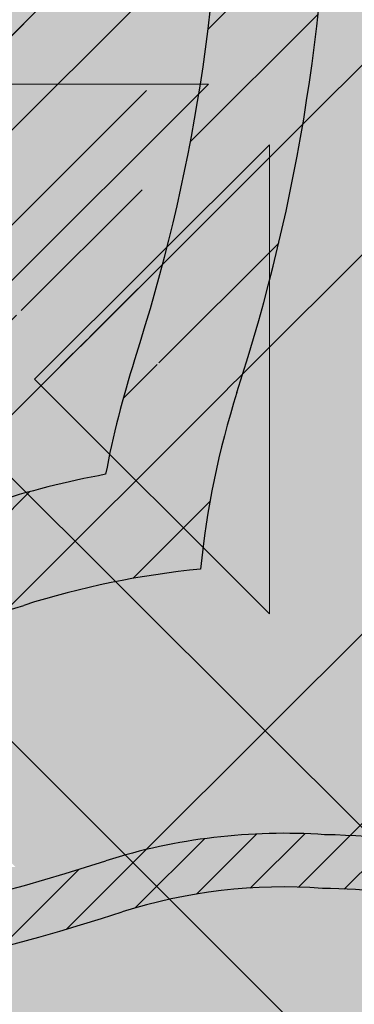
# Model space of a CAD drawing. Units: inches. Extents: x 844 to 2234, y 346 to 1084.
# Tile 10 of 93: x 1124.57 to 1125.562, y 688.258 to 691.183. Entities that reach past the tile are written whole.
import ezdxf

# ---------------------------------------------------------------- set-up
doc = ezdxf.new("R2010")
doc.units = ezdxf.units.IN
doc.header["$MEASUREMENT"] = 0
for name, color, linetype, lineweight in [('A-ANNO-DIMS', 2, 'Continuous', 18), ('furniture', 8, 'Continuous', 18), ('RA-AP-01$0$INT', 35, 'Continuous', 5)]:
    doc.layers.add(name, color=color, linetype=linetype, lineweight=lineweight)
doc.layers.add('RA-AP-01$0$FURN', color=3, linetype='Continuous')
doc.layers.add('RA-AP-01$0$WOOD', color=64, linetype='Continuous')
doc.styles.get("Standard").update_dxf_attribs({"font": 'arial.ttf'})
doc.dimstyles.get("Standard").update_dxf_attribs({"dimtxt": 6, "dimasz": 3, "dimexe": 0.18, "dimexo": 0.0625, "dimgap": 0.09, "dimtad": 0, "dimtih": 1, "dimtoh": 1, "dimdec": 1, "dimzin": 0, "dimdsep": 46, "dimlunit": 3, "dimtxsty": 'Standard', "dimblk": 'ARCHTICK', "dimcen": 0.09, "dimadec": 0, "dimazin": 0, "dimtfac": 1, "dimtdec": 1, "dimtofl": 0, "dimtmove": 0, "dimatfit": 3, "dimfxl": 1, "dimtolj": 1, "dimtzin": 0, "dimarcsym": 0})

# ---------------------------------------------------------------- blocks, each defined once
blk = doc.blocks.new('A$C18D01794')
at = {"layer": 'RA-AP-01$0$INT'}
h = blk.add_hatch(color=256, dxfattribs=at)
h.paths.add_polyline_path([(4.585917135068449, -6.356712009588271), (4.555206456959269, -6.35671200958746), (4.555206456959137, -6.387422687716308), (4.874495778835233, -6.706712009592356), (4.90520645695423, -6.676001331474049)])
h.paths.add_polyline_path([(5.255206456948813, -6.387422687716306), (5.255206456948682, -6.356712009605972), (5.224495778822613, -6.356712009605161), (4.905206456953498, -6.676001331474273), (4.935917135072151, -6.706712009592924)])
h.paths.add_polyline_path([(4.935917135072559, -6.706712009592068), (4.905206456953564, -6.737422687710376), (5.255206456951813, -7.087422687708613), (5.255206456951549, -7.026001331471008)])
h.paths.add_polyline_path([(4.555206456956399, -7.026001331471013), (4.555206456956134, -7.087422687708616), (4.905206456953821, -6.737422687710943), (4.874495778835166, -6.70671200959229)])
h = blk.add_hatch(color=256, dxfattribs=at)
h.paths.add_polyline_path([(4.585917135068448, -6.356712009588273), (4.614201406330596, -6.356712009589021), (4.668846067270487, -6.411356670531338), (4.723490728212344, -6.356712009591912), (4.771774999457151, -6.35671200959319), (4.826419660396886, -6.411356670535356), (4.862780050090322, -6.374996280843536), (4.844495778842715, -6.356712009595112), (4.862780050090411, -6.356712009595595), (4.905206456960182, -6.399138416468211), (4.947632863832445, -6.356712009597838), (4.965917135079675, -6.356712009598322), (4.947632863831759, -6.374996280845421), (4.983993253523576, -6.411356670538857), (5.038637914464627, -6.356712009600247), (5.08692218571208, -6.356712009601523), (5.141566846649976, -6.411356670541852), (5.196211507589851, -6.356712009604411), (5.224495778822615, -6.356712009605161), (4.905206456953975, -6.676001331473793)])
h.paths.add_polyline_path([(4.895206456956031, -6.637717060225675), (4.895206456958921, -6.528427738347902), (4.840561796018589, -6.583072399285802)], flags=16)
h.paths.add_polyline_path([(4.915206456955638, -6.637717060226121), (4.969851117895509, -6.583072399288678), (4.915206456957609, -6.528427738348344)], flags=16)
h.paths.add_polyline_path([(4.826419660395175, -6.568930263661755), (4.881064321335613, -6.514285602723745), (4.771774999456703, -6.514285602720857)], flags=16)
h.paths.add_polyline_path([(4.983993253519558, -6.568930263665262), (5.038637914460456, -6.514285602726792), (4.929348592581548, -6.514285602724816)], flags=16)
h.paths.add_polyline_path([(4.881064321336025, -6.494285602723742), (4.826419660397532, -6.439640941782821), (4.771774999457062, -6.494285602720859)], flags=16)
h.paths.add_polyline_path([(4.929348592582019, -6.494285602724817), (5.038637914460982, -6.494285602726792), (4.983993253522945, -6.439640941786327)], flags=16)
h.paths.add_polyline_path([(4.895206456960191, -6.480143467100443), (4.895206456962115, -6.407422687715913), (4.876922185715016, -6.389138416467584), (4.840561796021581, -6.425498806159401)], flags=16)
h.paths.add_polyline_path([(4.915206456958487, -6.480143467100889), (4.969851117899527, -6.425498806162279), (4.933490728206909, -6.389138416468043), (4.9152064569598, -6.40742268771434)], flags=16)
h.paths.add_polyline_path([(4.757632863832376, -6.480143467096812), (4.812277524772842, -6.425498806158772), (4.757632863834348, -6.370854145217844)], flags=16)
h.paths.add_polyline_path([(4.737632863832376, -6.480143467096286), (4.737632863834348, -6.370854145217375), (4.682988202893906, -6.425498806155385)], flags=16)
h.paths.add_polyline_path([(5.05278005008503, -6.480143467103376), (5.052780050087917, -6.370854145224413), (4.998135389146995, -6.425498806162908)], flags=16)
h.paths.add_polyline_path([(5.072780050085024, -6.480143467103744), (5.127424711025931, -6.42549880616527), (5.072780050087916, -6.370854145224832)], flags=16)
h.paths.add_polyline_path([(4.935917135072783, -6.706712009592292), (5.255206456948811, -6.387422687716309), (5.255206456948932, -6.415706958964177), (5.200561796010279, -6.470351619902839), (5.255206456949403, -6.524996280841948), (5.25520645694961, -6.5732805520894), (5.200561796009787, -6.627925213029239), (5.236922185702417, -6.664285602721864), (5.255206456949919, -6.646001331474357), (5.255206456949998, -6.664285602721898), (5.212780050078687, -6.706712009592262), (5.25520645695036, -6.749138416463932), (5.255206456950438, -6.767422687711313), (5.236922185702424, -6.749138416463297), (5.200561796009796, -6.785498806155928), (5.255206456950753, -6.840143467096874), (5.25520645695096, -6.888427738341682), (5.200561796010322, -6.943072399282328), (5.255206456951428, -6.997717060223427), (5.255206456951547, -7.026001331471006)])
h.paths.add_polyline_path([(5.042988202883395, -6.785498806155427), (5.097632863823085, -6.840143467095101), (5.097632863822622, -6.730854145216193)], flags=16)
h.paths.add_polyline_path([(5.028846067259663, -6.771356670531693), (5.083490728198774, -6.716712009592573), (4.974201406321001, -6.716712009593042)], flags=16)
h.paths.add_polyline_path([(5.117632863823087, -6.840143467095186), (5.172277524762331, -6.785498806155926), (5.11763286382262, -6.730854145216225)], flags=16)
h.paths.add_polyline_path([(5.08349072819877, -6.696712009593886), (5.028846067259652, -6.642067348654775), (4.974201406320998, -6.696712009593438)], flags=16)
h.paths.add_polyline_path([(5.131774999446817, -6.854285602718917), (5.186419660386065, -6.799640941779662), (5.241064321325782, -6.854285602719365)], flags=17)
h.paths.add_polyline_path([(5.131774999446228, -6.716712009592374), (5.186419660386065, -6.771356670532194), (5.222780050079488, -6.734996280838764), (5.204495778832781, -6.716712009592063)], flags=16)
h.paths.add_polyline_path([(5.097632863822613, -6.682569873970264), (5.097632863823061, -6.573280552091354), (5.042988202883383, -6.627925213031044)], flags=16)
h.paths.add_polyline_path([(5.131774999446899, -6.874285602718915), (5.241064321325809, -6.874285602719364), (5.186419660386591, -6.928930263658598)], flags=17)
h.paths.add_polyline_path([(5.131774999446226, -6.696712009594078), (5.204495778830767, -6.696712009594374), (5.22278005007868, -6.67842773834687), (5.186419660386049, -6.642067348654249)], flags=16)
h.paths.add_polyline_path([(5.11763286382262, -6.682569873970225), (5.17227752476232, -6.627925213030515), (5.117632863823064, -6.573280552091267)], flags=16)
h.paths.add_polyline_path([(5.186419660386069, -6.613783077405491), (5.241064321325754, -6.559138416465795), (5.131774999446791, -6.559138416466263)], flags=16)
h.paths.add_polyline_path([(5.131774999446872, -6.539138416466263), (5.24106432132578, -6.539138416465794), (5.186419660386554, -6.484493755526573)], flags=16)
h.paths.add_polyline_path([(5.255206456951811, -7.08742268770861), (5.255206456951895, -7.106712009588038), (4.555206456956052, -7.106712009588038), (4.555206456956136, -7.087422687708617), (4.905206456953973, -6.737422687710788)])
h.paths.add_polyline_path([(4.983993253513404, -6.8444937555241), (4.92934859257295, -6.899138416462108), (5.03863791445186, -6.899138416465014)], flags=16)
h.paths.add_polyline_path([(4.969851117889988, -6.83035161990006), (4.915206456952556, -6.775706958960171), (4.915206456949648, -6.884996280837944)], flags=16)
h.paths.add_polyline_path([(4.929348592572535, -6.919138416462105), (4.983993253511019, -6.973783077403037), (5.038637914451496, -6.919138416465012)], flags=16)
h.paths.add_polyline_path([(5.052780050074912, -6.93328055208906), (4.998135389134438, -6.987925213027088), (5.052780050072919, -7.042569873968025)], flags=16)
h.paths.add_polyline_path([(5.07278005007491, -6.933280552089588), (5.072780050072918, -7.042569873968497), (5.127424711013374, -6.987925213030498)], flags=16)
h.paths.add_polyline_path([(4.89520645695295, -6.775706958959721), (4.840561796013067, -6.830351619897157), (4.895206456950961, -6.884996280837494)], flags=16)
h.paths.add_polyline_path([(4.915206456948365, -6.933280552085403), (4.915206456946434, -7.006001331471951), (4.933490728192729, -7.024285602719066), (4.969851117886972, -6.987925213026453)], flags=16)
h.paths.add_polyline_path([(4.881064321327021, -6.899138416461022), (4.82641966038902, -6.84449375552057), (4.771774999448108, -6.899138416459029)], flags=16)
h.paths.add_polyline_path([(4.895206456950073, -6.933280552084951), (4.840561796009022, -6.987925213023558), (4.876922185700835, -7.024285602716997), (4.895206456948749, -7.006001331469487)], flags=16)
h.paths.add_polyline_path([(4.983993253510392, -7.0020673486505), (4.947632863816944, -7.038427738342319), (4.965917135064043, -7.05671200959023), (5.038637914448995, -7.056712009591555)], flags=16)
h.paths.add_polyline_path([(4.881064321326543, -6.91913841646102), (4.771774999447578, -6.919138416459031), (4.826419660385607, -6.973783077399508)], flags=16)
h.paths.add_polyline_path([(4.905206456946447, -7.014285602717636), (4.862780050074785, -7.056712009588352), (4.947632863816685, -7.056712009589775)], flags=16)
h.paths.add_polyline_path([(5.14156684663679, -7.002067348654549), (5.086922185696452, -7.056712009592438), (5.196211507574223, -7.056712009594425)], flags=16)
h.paths.add_polyline_path([(4.8264196603837, -7.002067348646972), (4.771774999442643, -7.056712009585575), (4.8444957788276, -7.056712009587508), (4.862780050075511, -7.038427738340416)], flags=16)
h.paths.add_polyline_path([(4.812277524760289, -6.98792521302292), (4.757632863822258, -6.933280552082447), (4.757632863819352, -7.042569873961408)], flags=16)
h.paths.add_polyline_path([(4.73763286382226, -6.933280552082079), (4.682988202881349, -6.987925213020536), (4.737632863819352, -7.04256987396099)], flags=16)
h.paths.add_polyline_path([(4.723490728195188, -7.056712009584289), (4.668846067257299, -7.002067348643949), (4.614201406317417, -7.056712009581383)], flags=16)
h.paths.add_polyline_path([(4.597632863829262, -6.706712009592262), (4.555206456957951, -6.664285602721896), (4.555206456958029, -6.646001331474357), (4.573490728205535, -6.664285602721864), (4.609851117898167, -6.627925213029238), (4.555206456958338, -6.573280552089402), (4.555206456958546, -6.524996280841952), (4.60985111789767, -6.470351619902839), (4.555206456959015, -6.415706958964177), (4.555206456959138, -6.387422687716309), (4.874495778835167, -6.70671200959229), (4.5552064569564, -7.026001331471015), (4.555206456956523, -6.997717060223433), (4.609851117897629, -6.94307239928233), (4.555206456956988, -6.888427738341681), (4.555206456957198, -6.840143467096881), (4.609851117898153, -6.78549880615593), (4.573490728205528, -6.749138416463297), (4.555206456957507, -6.76742268771132), (4.555206456957585, -6.749138416463933)])
h.paths.add_polyline_path([(4.712780050085332, -6.730854145216195), (4.712780050084863, -6.840143467095105), (4.767424711024555, -6.785498806155427)], flags=16)
h.paths.add_polyline_path([(4.726922185709173, -6.716712009592573), (4.781566846648288, -6.771356670531693), (4.836211507586949, -6.716712009593043)], flags=16)
h.paths.add_polyline_path([(4.692780050085327, -6.730854145216225), (4.638135389145619, -6.785498806155928), (4.692780050084865, -6.840143467095185)], flags=16)
h.paths.add_polyline_path([(4.726922185709182, -6.696712009593886), (4.836211507586949, -6.696712009593436), (4.7815668466483, -6.642067348654773)], flags=16)
h.paths.add_polyline_path([(4.678637914461726, -6.71671200959237), (4.605917135075169, -6.716712009592063), (4.587632863828464, -6.734996280838766), (4.623993253521887, -6.771356670532195)], flags=16)
h.paths.add_polyline_path([(4.712780050085336, -6.68256987397026), (4.767424711024568, -6.627925213031042), (4.71278005008489, -6.573280552091352)], flags=16)
h.paths.add_polyline_path([(4.678637914461726, -6.696712009594076), (4.623993253521899, -6.642067348654247), (4.587632863829271, -6.67842773834687), (4.605917135077185, -6.696712009594376)], flags=16)
h.paths.add_polyline_path([(4.692780050085336, -6.682569873970228), (4.692780050084889, -6.573280552091267), (4.638135389145632, -6.627925213030515)], flags=16)
h.paths.add_polyline_path([(4.623993253521885, -6.799640941779662), (4.678637914461131, -6.854285602718915), (4.56934859258217, -6.854285602719365)], flags=17)
h.paths.add_polyline_path([(4.623993253521901, -6.613783077405509), (4.678637914461158, -6.559138416466263), (4.569348592582195, -6.559138416465795)], flags=16)
h.paths.add_polyline_path([(4.678637914461051, -6.874285602718915), (4.623993253521361, -6.928930263658598), (4.569348592582143, -6.874285602719364)], flags=17)
h.paths.add_polyline_path([(4.678637914461076, -6.539138416466263), (4.623993253521399, -6.484493755526573), (4.569348592582167, -6.539138416465796)], flags=16)
h = blk.add_hatch(color=256, dxfattribs=at)
h.paths.add_polyline_path([(5.028846067259997, -6.642067348655121), (4.974201406321342, -6.696712009593783), (5.083490728199115, -6.69671200959423)])
h.paths.add_polyline_path([(4.974201406321344, -6.716712009593388), (5.028846067260004, -6.771356670532039), (5.083490728199117, -6.716712009592919)])
h.paths.add_polyline_path([(5.042988202883738, -6.785498806155768), (5.097632863823428, -6.840143467095449), (5.097632863822963, -6.73085414521654)])
h.paths.add_polyline_path([(5.117632863822961, -6.730854145216568), (5.117632863823428, -6.840143467095531), (5.172277524762674, -6.785498806156272)])
h.paths.add_polyline_path([(5.131774999446572, -6.716712009592718), (5.186419660386406, -6.77135667053254), (5.222780050079831, -6.734996280839116), (5.204495778833122, -6.716712009592409)])
h.paths.add_polyline_path([(5.236922185702764, -6.749138416463644), (5.200561796010139, -6.785498806156274), (5.255206456949971, -6.840143467096101), (5.255206456950271, -6.76742268771115)])
h.paths.add_polyline_path([(5.186419660386412, -6.799640941780006), (5.131774999447164, -6.854285602719262), (5.241064321326123, -6.854285602719711)])
h.paths.add_polyline_path([(5.131774999447238, -6.874285602719261), (5.186419660386934, -6.928930263658944), (5.241064321326153, -6.874285602719709)])
h.paths.add_polyline_path([(5.200561796010663, -6.943072399282675), (5.255206456949324, -6.997717060221329), (5.255206456949777, -6.888427738343558)])
h.paths.add_polyline_path([(5.21278005007903, -6.706712009592607), (5.255206456950223, -6.749138416463798), (5.255206456950696, -6.664285602721891)])
h.paths.add_polyline_path([(5.13177499944657, -6.696712009594424), (5.204495778831106, -6.696712009594723), (5.222780050079024, -6.678427738347219), (5.186419660386397, -6.642067348654592)])
h.paths.add_polyline_path([(5.117632863823405, -6.573280552091611), (5.117632863822955, -6.682569873970578), (5.172277524762665, -6.627925213030859)])
h.paths.add_polyline_path([(5.042988202883727, -6.627925213031387), (5.097632863822957, -6.682569873970603), (5.097632863823407, -6.573280552091697)])
h.paths.add_polyline_path([(5.131774999447135, -6.559138416466609), (5.186419660386394, -6.613783077405857), (5.241064321326097, -6.559138416466144)])
h.paths.add_polyline_path([(5.200561796010128, -6.627925213029584), (5.236922185702758, -6.664285602722211), (5.255206456950264, -6.646001331474705), (5.255206456949948, -6.573280552089752)])
h.paths.add_polyline_path([(5.186419660386895, -6.484493755526919), (5.131774999447213, -6.539138416466609), (5.241064321326127, -6.539138416466142)])
h.paths.add_polyline_path([(5.200561796010624, -6.470351619903183), (5.255206456949745, -6.524996280842298), (5.255206456949276, -6.415706958964523)])
for p, q in [((4.905206456953975, -6.676001331473793), (5.224495778822613, -6.356712009605161)), ((4.935917135072783, -6.706712009592292), (5.255206456948813, -6.387422687716307)), ((5.042988202883385, -6.627925213031041), (5.097632863823062, -6.573280552091352)), ((5.097632863823062, -6.573280552091352), (5.097632863822615, -6.682569873970262)), ((5.097632863822615, -6.682569873970262), (5.042988202883383, -6.627925213031042)), ((5.083490728198769, -6.696712009593882), (5.028846067259652, -6.642067348654775)), ((5.08349072819877, -6.696712009593886), (4.974201406320999, -6.696712009593436))]:
    blk.add_line(p, q, dxfattribs=at)
blk = doc.blocks.new('A$C32926AE1')
at = {"layer": 'RA-AP-01$0$FURN'}
h = blk.add_hatch(dxfattribs=at)
h.set_pattern_fill('ANSI31', color=256, scale=0.1, style=0)
h.set_pattern_definition([(45, (0, 0), (-0.0088388347648318, 0.0088388347648318), [])])
edge = h.paths.add_edge_path(flags=16)
edge.add_arc((4.904771284329206, 4.246793130718756), 0.2603971832811541, 75.22398030683196, 104.7760196931204)
edge.add_arc((4.904771284329206, 4.246793130718756), 0.2603971832811541, 75.223980306832, 104.77601969312039, ccw=False)
edge = h.paths.add_edge_path(flags=16)
edge.add_arc((4.904771284329206, 4.067062675376612), 0.2603971832811541, 255.2239803068796, 284.776019693168)
edge.add_arc((4.904771284329206, 4.067062675376612), 0.2603971832811541, 255.22398030687958, 284.77601969316805, ccw=False)
edge = h.paths.add_edge_path(flags=0)
edge.add_arc((4.904771284329206, 4.067062675376612), 0.2603971832811541, 255.2239803068796, 284.776019693168)
edge.add_arc((4.904771284329206, 4.067062675376612), 0.2603971832811541, 255.22398030687958, 284.77601969316805, ccw=False)
edge = h.paths.add_edge_path(flags=0)
edge.add_arc((4.904771284329206, 4.067062675376612), 0.2603971832811541, 255.2239803068796, 284.776019693168)
edge.add_arc((4.904771284329206, 4.067062675376612), 0.2603971832811541, 255.22398030687958, 284.77601969316805, ccw=False)
edge = h.paths.add_edge_path()
edge.add_arc((4.604388392048174, 4.588829985554312), 0.1599999999999918, 342.3781640246255, 354.4317409793762)
edge.add_arc((5.090145208887507, 4.43216705527679), 0.3503971832811637, 162.0091218307731, 180.3186872093483)
edge.add_arc((5.205154176610243, 4.588829985554953), 0.1599999999999917, 185.5682590208461, 197.6218359767349)
edge.add_arc((4.904771284329229, 4.246793130718735), 0.3503971832811761, 72.00912183053516, 107.9908781690354)
edge.add_arc((9.535952835716557, 4.28682295566602), 4.798342501046485, 178.2875002453811, 181.5576802719453)
edge.add_arc((4.719397359771122, 4.43216705527679), 0.3503971832811637, 359.6813127906516, 377.9908781692269)
edge.add_arc((9.535967292294904, 4.286822350292874), 4.778371420254705, 178.2965938931842, 181.5667745797229)
edge.add_arc((4.719397359771122, 4.43216705527679), 0.3303971832811637, 359.6813127906516, 377.9908781692269)
edge.add_arc((0.2735752763637294, 4.286822350292874), 4.7783714202547, 358.4332254202771, 361.7034061068158)
edge.add_arc((5.061434214606998, 4.732549947558029), 0.1600000000000254, 252.3781640250584, 264.4317409792362)
edge.add_arc((4.748108354051257, 4.732549947558012), 0.1600000000000541, 275.5682590208426, 287.6218359759532)
edge.add_arc((4.604388392048115, 4.588829985554317), 0.1800000000000505, 342.3567572500182, 349.3735009646207)
edge.add_arc((5.205154176610254, 4.588829985554976), 0.1800000000000069, 190.6264990356027, 197.6432427513933)
edge.add_arc((5.061434214607106, 4.732549947558013), 0.1800000000000424, 252.3567572496606, 259.3735009644582)
edge.add_arc((4.904771284329208, 4.246793130718737), 0.3303971832811676, 71.99844483668534, 108.0015551637021)
edge.add_arc((4.748108354051414, 4.732549947558045), 0.1800000000000547, 280.6264990355479, 287.6432427495938)
edge.add_arc((5.090145208887514, 4.432167055276789), 0.2803971832811691, 162.8706300666893, 180.816523289902)
edge.add_arc((4.719397359771136, 4.432167055276689), 0.2803971832811534, 359.183476710103, 377.1293699333214)
edge.add_arc((4.904771284329222, 4.246793130718737), 0.2803971832811769, 72.87063006672916, 107.1293699332334)
edge.add_arc((5.090145208887522, 4.432167055276788), 0.2603971832811776, 165.2239803068007, 180.9953123810312)
edge.add_arc((4.719397359771141, 4.432167055276699), 0.2603971832811458, 359.0046876189768, 374.7760196932087)
edge.add_arc((5.090145208887507, 4.43216705527679), 0.3303971832811637, 162.0091218307731, 180.3186872093483)
edge.add_arc((9.53595427642584, 4.285015535491528), 4.728345371032053, 178.265043920078, 181.5679956281801)
edge.add_arc((0.2735882922327999, 4.285015535491582), 4.728345371032045, 358.4320043718193, 361.7349560799204)
edge.add_arc((9.535953591267507, 4.284458026472751), 4.708343996644348, 178.2573054306777, 181.5704995759608)
edge.add_arc((0.273588977391114, 4.284458026472785), 4.708343996644358, 358.4295004240388, 361.7426945693213)
edge.add_arc((0.2735889773911131, 4.029397779622582), 4.708343996644359, 358.2573054306787, 361.5704995759613)
edge.add_arc((9.535953591267518, 4.029397779622618), 4.708343996644359, 178.4295004240391, 181.7426945693223)
edge.add_arc((0.2735882922327901, 4.028840270603786), 4.728345371032054, 358.2650439200796, 361.5679956281808)
edge.add_arc((9.53595427642584, 4.028840270603841), 4.728345371032054, 178.4320043718199, 181.7349560799219)
edge.add_arc((0.2735752763637302, 4.027033455802493), 4.778371420254699, 358.2965938931842, 361.5667745797229)
edge.add_arc((4.719397359771122, 3.881688750818578), 0.3303971832811637, 342.0091218307731, 360.3186872093484)
edge.add_arc((5.090145208887507, 3.881688750818578), 0.3303971832811637, 179.6813127906516, 197.9908781692269)
edge.add_arc((9.535967292294904, 4.027033455802493), 4.778371420254705, 178.433225420277, 181.7034061068158)
edge.add_arc((4.719397359771122, 3.881688750818578), 0.3503971832811637, 342.0091218307731, 360.3186872093484)
edge.add_arc((9.53595283571655, 4.027032850429349), 4.79834250104648, 178.4423197280546, 181.7124997546188)
edge.add_arc((4.719397359771141, 3.881688750818669), 0.2603971832811458, 345.2239803067913, 360.9953123810232)
edge.add_arc((5.090145208887522, 3.88168875081858), 0.2603971832811776, 179.0046876189687, 194.7760196931993)
edge.add_arc((4.904771284329222, 4.067062675376631), 0.2803971832811769, 252.8706300667665, 287.1293699332708)
edge.add_arc((4.719397359771136, 3.881688750818678), 0.2803971832811534, 342.8706300666787, 360.8165232898969)
edge.add_arc((5.090145208887514, 3.881688750818579), 0.2803971832811691, 179.183476710098, 197.1293699333106)
edge.add_arc((4.748108354051414, 3.581305858537323), 0.1800000000000547, 72.3567572504062, 79.37350096445199)
edge.add_arc((4.904771284329208, 4.067062675376631), 0.3303971832811676, 251.9984448362979, 288.0015551633146)
edge.add_arc((5.061434214607106, 3.581305858537355), 0.1800000000000424, 100.6264990355418, 107.6432427503394)
edge.add_arc((5.205154176610254, 3.725025820540392), 0.1800000000000069, 162.3567572486066, 169.3735009643972)
edge.add_arc((4.604388392048115, 3.725025820541051), 0.1800000000000505, 10.62649903537925, 17.64324274998182)
edge.add_arc((4.748108354051257, 3.581305858537356), 0.1600000000000541, 72.37816402404681, 84.43174097915735)
edge.add_arc((4.904771284329229, 4.067062675376632), 0.3503971832811761, 252.0091218309645, 287.9908781694648)
edge.add_arc((5.061434214606998, 3.581305858537339), 0.1600000000000254, 95.56825902076373, 107.6218359749416)
edge.add_arc((5.205154176610243, 3.725025820540414), 0.1599999999999917, 162.3781640232651, 174.4317409791539)
edge.add_arc((5.090145208887507, 3.881688750818578), 0.3503971832811637, 179.6813127906516, 197.9908781692269)
edge.add_arc((4.604388392048174, 3.725025820541056), 0.1599999999999918, 5.568259020623824, 17.62183597537444)
edge.add_arc((0.2735897329420762, 4.28682295566602), 4.798342501046482, 358.4423197280547, 361.7124997546188)
edge.add_arc((0.2735897329420691, 4.027032850429348), 4.798342501046489, 358.2875002453812, 361.5576802719453)
at = {"layer": 'RA-AP-01$0$WOOD'}
h = blk.add_hatch(color=256, dxfattribs=at)
h.dxf.hatch_style = 1
h.paths.add_polyline_path([(5.157430609644524, 4.573483066760929, -0.1009492694046607), (5.155401577623758, 4.593365984175333, -0.1842662638101597), (5.172249623284174, 4.638795604568598, 0.2056608120311276), (5.179560981299304, 4.661316324430096, 0.3614336704623542), (5.134352340494423, 4.706524965234944, 0.2056608120311297), (5.111831620632933, 4.699213607219793, -0.1842662638101113), (5.066402000239693, 4.682365561559342, -0.1055311479399994), (5.045656153913092, 4.68467289944697, 0.1567636581983829), (4.763886414745334, 4.684672899446966, -0.1055311479399895), (4.743140568418733, 4.68236556155934, -0.1842662638100833), (4.6977109480255, 4.69921360721979, 0.2056608120302612), (4.675190228164109, 4.706524965234949, 0.3614336704708441), (4.629981587358889, 4.66131632442871, 0.2056608120245944), (4.637292945374126, 4.638795604567974, -0.1842662638101024), (4.654140991034615, 4.59336598417475, -0.1009492694055169), (4.652111959013835, 4.573483066760181, 0.021410119221476), (4.629748025606143, 4.156712009541676, 0.0214101192214795), (4.652111959013809, 3.739940952323101, -0.1009492694059586), (4.654140991034615, 3.720058034908448, -0.1842662638100975), (4.637292945374126, 3.674628414515226, 0.2056608120245705), (4.629981587358889, 3.652107694654492, 0.3614336704708879), (4.675190228164113, 3.606899053848249, 0.2056608120302384), (4.697710948025501, 3.614210411863408, -0.1842662638100995), (4.743140568418738, 3.63105845752386, -0.1055311479402541), (4.763886414745388, 3.628751119636215, 0.1567636581983776), (5.045656153913137, 3.628751119636244, -0.1055311479397538), (5.066402000239692, 3.631058457523857, -0.1842662638101067), (5.111831620632931, 3.614210411863407, 0.2056608120310924), (5.134352340494417, 3.606899053848256, 0.3614336704624001), (5.179560981299307, 3.652107694653103, 0.2056608120311314), (5.172249623284175, 3.6746284145146, -0.1842662638101402), (5.155401577623758, 3.72005803490786, -0.1009492694051366), (5.15743060964455, 3.739940952322354, 0.0214101192215073), (5.179794543052287, 4.156712009541468, 0.0214101192215252)])
h.paths.add_polyline_path([(4.639748609479751, 4.156712009541513, 0.0213537860821624), (4.661970494867118, 3.741887061152232, -0.094075836301374), (4.664143710413708, 3.7196126951003, -0.1824818158568985), (4.644813765429836, 3.668037719127816, 0.2056608120245319), (4.639939526753007, 3.653023905887301, 0.3614336704710246), (4.676106439397173, 3.616856993242342, 0.2056608120302234), (4.691120252638095, 3.621731231919122, -0.1824818158602558), (4.742695228611606, 3.641061176902986, -0.1029891339458722), (4.766991894714349, 3.638256818950944, 0.156709409989566), (5.042550673941472, 3.638256818950105, -0.102989133958497), (5.066847340047078, 3.641061176902949, -0.1824818158594995), (5.118422316020358, 3.621731231919103, 0.2056608120311416), (5.133436129261316, 3.616856993242346, 0.3614336704621468), (5.169603041905217, 3.653023905886178, 0.2056608120310986), (5.164728803228477, 3.668037719127177, -0.1824818158565612), (5.145398858244737, 3.719612695099578, -0.0940758363009313), (5.147572073791232, 3.741887061151398, 0.0213537860822023), (5.169793959178681, 4.156712009541451, 0.0213537860822226), (5.147572073791203, 4.571536957931898, -0.0940758363005034), (5.145398858244737, 4.59381132398362, -0.1824818158565587), (5.164728803228476, 4.645386299956021, 0.2056608120311045), (5.169603041905216, 4.66040011319702, 0.3614336704621845), (5.133436129261313, 4.696567025840856, 0.2056608120310773), (5.118422316020359, 4.691692787164098, -0.182481815859508), (5.066847340047078, 4.67236284218025, -0.1029891339584606), (5.04255067394148, 4.675167200133092, 0.156709409989566), (4.766991894714357, 4.675167200132257, -0.1029891339458842), (4.742695228611611, 4.672362842180213, -0.1824818158602725), (4.691120252638095, 4.691692787164077, 0.2056608120302152), (4.676106439397174, 4.696567025840858, 0.3614336704710363), (4.639939526753005, 4.660400113195899, 0.2056608120245495), (4.644813765429837, 4.645386299955384, -0.1824818158568934), (4.664143710413708, 4.593811323982902, -0.0940758363009187), (4.661970494867149, 4.571536957931074, 0.021353786082177)], flags=16)
h.paths.add_polyline_path([(5.129794543052235, 4.432167055276933, -0.0141661062790638), (5.130152669293814, 4.156927903047693, -0.0141661062790647), (5.129794543052234, 3.881688750818433, -0.0785247771143638), (5.10979738006795, 3.755143611847103, 0.0945969212073497), (5.105408519571111, 3.717898134952927, 0.1043170707844957), (5.116074640131521, 3.670385395016088, 0.1043170707864965), (5.068561900193738, 3.681051515576561, 0.09459692119553), (5.031316423304057, 3.676662655080835, -0.1580239521427272), (4.778226145355827, 3.676662655080367, 0.0945969211986668), (4.740980668464973, 3.681051515576592, 0.1043170707882822), (4.693467928526415, 3.670385395015844, 0.1043170707867916), (4.704134049087309, 3.717898134953662, 0.0945969211972894), (4.69974518859162, 3.755143611844042, -0.0785247771163196), (4.679748025606343, 3.881688750818406, -0.0141661062790663), (4.679389899364763, 4.156927903047693, -0.0141661062790672), (4.679748025606343, 4.432167055276998, -0.0785247771163064), (4.699745188591625, 4.55871219425134, 0.094596921197333), (4.704134049087308, 4.595957671141738, 0.1043170707867205), (4.693467928526416, 4.643470411079523, 0.1043170707882628), (4.740980668464965, 4.632804290518776, 0.0945969211988114), (4.778226145355874, 4.637193151015016, -0.158023952142669), (5.031316423304015, 4.637193151014546, 0.0945969211956361), (5.068561900193736, 4.632804290518806, 0.1043170707864979), (5.11607464013152, 4.643470411079278, 0.1043170707844617), (5.105408519571112, 4.595957671142455, 0.0945969212074597), (5.109797380067959, 4.558712194248236, -0.0785247771143467)], flags=0)
h.paths.add_polyline_path([(5.119794532311105, 4.432259799204851, -0.0142000800617244), (5.120156169157484, 4.156927903047701, -0.0142000800617277), (5.119794532311105, 3.881596006890482, -0.0784894509520253), (5.100273383573699, 3.758192358677797, 0.0940138827242913), (5.095413455884425, 3.717477693979438, 0.0606271852308753), (5.099615656341024, 3.686844378806616, 0.0606271852322524), (5.068982341167493, 3.691046579263239, 0.0940138827010453), (5.028267676478798, 3.686186651576848, -0.1580706864508061), (4.781274892180912, 3.686186651576435, 0.0940138827026903), (4.740560227491556, 3.691046579263279, 0.0606271852339895), (4.709926912317155, 3.686844378806508, 0.0606271852329405), (4.714129112773991, 3.717477693980356, 0.094013882701304), (4.709269185087677, 3.758192358669163, -0.0784894509577193), (4.689748036347473, 3.881596006890469, -0.014200080061729), (4.689386399501094, 4.156927903047709, -0.0142000800617217), (4.689748036347473, 4.432259799204808, -0.078489450957724), (4.709269185087651, 4.555663447426125, 0.0940138827014585), (4.714129112773992, 4.596378112114996, 0.0606271852329731), (4.709926912317154, 4.62701142728886, 0.0606271852340196), (4.74056022749157, 4.622809226832087, 0.0940138827024997), (4.781274892180847, 4.627669154518912, -0.1580706864508359), (5.028267676478777, 4.627669154518526, 0.0940138827010946), (5.068982341167492, 4.622809226832129, 0.060627185232254), (5.099615656341024, 4.627011427288751, 0.0606271852308727), (5.095413455884425, 4.59637811211593, 0.0940138827241088), (5.100273383573675, 4.555663447417647, -0.0784894509520978)], flags=0)
h.paths.add_polyline_path([(5.06978912287499, 4.430218106756144, -0.014241683694547), (5.070173729147532, 4.156927903047672, -0.0142416836945458), (5.06978912287499, 3.883637699339223, -0.0800609523125196), (5.052662118612511, 3.773463122773442, 0.0526421978001116), (5.04590916754064, 3.740550867606997, 0.0526421977992423), (5.012996912374707, 3.73379791653534, -0.1583028414718258), (4.796545656286308, 3.73379791653451, 0.0526421978034211), (4.763633401117837, 3.740550867607021, 0.0526421978018622), (4.756880450045755, 3.773463122774558, -0.0800609523117106), (4.739753445783639, 3.883637699339268, -0.0142416836945435), (4.739368839511098, 4.156927903047671, -0.0142416836945477), (4.739753445783639, 4.430218106756155, -0.0800609523116345), (4.75688045004574, 4.540392683320762, 0.052642197801941), (4.763633401117837, 4.573304938488346, 0.0526421978035071), (4.796545656286361, 4.580057889560873, -0.1583028414717561), (5.012996912374669, 4.580057889560039, 0.0526421977993048), (5.04590916754064, 4.57330493848837, 0.0526421978002057), (5.052662118612529, 4.540392683321868, -0.080060952312477)], flags=0)
h.paths.add_polyline_path([(5.049789715110557, 4.43038092723357, -0.0143097550741839), (5.05018085590259, 4.156927903047715, -0.0143097550741854), (5.049789715110558, 3.883474878861827, -0.0800685599149176), (5.03362098255317, 3.779581877367999, 0.0306258898956367), (5.028241146483733, 3.758218888663947, 0.0306258898977031), (5.006878157778253, 3.75283905259408, -0.1583983521624096), (4.802664410878162, 3.752839052594731, 0.0306258898946014), (4.781301422174808, 3.758218888663924, 0.0306258898967912), (4.775921586105202, 3.779581877368794, -0.080068559914251), (4.759752853548071, 3.883474878861786, -0.0143097550741854), (4.759361712756037, 4.156927903047671, -0.0143097550741854), (4.759752853548071, 4.430380927233557, -0.0800685599142479), (4.775921586105193, 4.534273928726546, 0.0306258898968306), (4.781301422174808, 4.555636917431444, 0.0306258898945754), (4.802664410878143, 4.561016753500631, -0.1583983521624168), (5.006878157778244, 4.561016753501291, 0.0306258898977177), (5.028241146483733, 4.555636917431421, 0.0306258898958182), (5.03362098255321, 4.534273928727244, -0.080068559914796)], flags=0)
h.paths.add_polyline_path([(4.999766070382627, 4.428171244713864, -0.0143443147609634), (5.000198441819402, 4.156927903047689, -0.0143443147609612), (4.999766070382627, 3.885684561381556, -0.0784641635803329), (4.987356730658798, 3.799103304488872, -0.1506053783831347), (4.822185837999821, 3.79910330448882, -0.0784641635803318), (4.809776498276007, 3.885684561381509, -0.014344314760963), (4.809344126839227, 4.156927903047677, -0.0143443147609645), (4.809776498276007, 4.428171244713873, -0.0784641635803192), (4.822185837999822, 4.514752501606549, -0.1506053783831338), (4.987356730658798, 4.514752501606494, -0.078464163580285)], flags=0)
h.paths.add_polyline_path([(4.979755254238824, 4.42764379880488, -0.0143772539198268), (4.980205517789977, 4.156927903047693, -0.0143772539198275), (4.979755254238824, 3.886212007290489, -0.0689242507424422), (4.971183264704897, 3.815276770442801, -0.1296645318904179), (4.838359303953726, 3.815276770442746, -0.0689242507424186), (4.829787314419809, 3.886212007290419, -0.0143772539198292), (4.829337050868653, 4.156927903047653, -0.0143772539198325), (4.829787314419809, 4.427643798804946, -0.0689242507424211), (4.838359303953725, 4.498579035652621, -0.1296645318904187), (4.971183264704897, 4.498579035652565, -0.0689242507424401)], flags=0)
h = blk.add_hatch(color=256, dxfattribs=at)
h.dxf.hatch_style = 1
h.paths.add_polyline_path([(5.145398858244737, 4.59381132398362, -0.1824818158565616), (5.164728803228476, 4.645386299956021, 0.2056608120311045), (5.169603041905216, 4.66040011319702, 0.3614336704621845), (5.133436129261313, 4.696567025840856, 0.2056608120310773), (5.118422316020359, 4.691692787164098, -0.182481815859508), (5.066847340047078, 4.67236284218025, -0.1029891339584606), (5.04255067394148, 4.675167200133092, 0.156709409989566), (4.766991894714357, 4.675167200132257, -0.1029891339458842), (4.742695228611611, 4.672362842180213, -0.1824818158602725), (4.691120252638095, 4.691692787164077, 0.2056608120302152), (4.676106439397174, 4.696567025840858, 0.3614336704710363), (4.639939526753005, 4.660400113195899, 0.2056608120245495), (4.644813765429837, 4.645386299955384, -0.1824818158568934), (4.664143710413708, 4.593811323982902, -0.0940758363009187), (4.661970494867149, 4.571536957931074, 0.0213537860821772), (4.639748609479751, 4.156712009541507, 0.0213537860821625), (4.661970494867119, 3.741887061152226, -0.0940758363013071), (4.664143710413708, 3.719612695100309, -0.1824818158569294), (4.644813765429836, 3.668037719127816, 0.2056608120245319), (4.639939526753007, 3.653023905887301, 0.3614336704710246), (4.676106439397173, 3.616856993242342, 0.2056608120302234), (4.691120252638095, 3.621731231919122, -0.1824818158602558), (4.742695228611606, 3.641061176902986, -0.1029891339458722), (4.766991894714349, 3.638256818950944, 0.156709409989566), (5.042550673941472, 3.638256818950105, -0.102989133958497), (5.066847340047078, 3.641061176902949, -0.1824818158594995), (5.118422316020358, 3.621731231919103, 0.2056608120311416), (5.133436129261316, 3.616856993242346, 0.3614336704621468), (5.169603041905217, 3.653023905886178, 0.2056608120310986), (5.164728803228477, 3.668037719127177, -0.1824818158565612), (5.145398858244737, 3.719612695099578, -0.0940758363009313), (5.147572073791232, 3.741887061151398, 0.0213537860822023), (5.169793959178681, 4.156712009541451, 0.0213537860822226), (5.147572073791203, 4.571536957931898, -0.0940758363004996)])
h.paths.add_polyline_path([(5.109797380067958, 4.55871219424824, -0.0785247771143472), (5.129794543052234, 4.432167055276936, -0.0141661062790644), (5.130152669293814, 4.156927903047685, -0.014166106279066), (5.129794543052234, 3.881688750818401, -0.0785247771143517), (5.109797380067946, 3.755143611847092, 0.0945969212073132), (5.105408519571111, 3.717898134952929, 0.1043170707844995), (5.116074640131521, 3.670385395016088, 0.1043170707864965), (5.068561900193738, 3.681051515576561, 0.09459692119553), (5.031316423304057, 3.676662655080835, -0.1580239521427272), (4.778226145355827, 3.676662655080367, 0.0945969211986668), (4.740980668464973, 3.681051515576592, 0.1043170707882822), (4.693467928526415, 3.670385395015844, 0.1043170707867916), (4.704134049087309, 3.717898134953662, 0.0945969211972894), (4.69974518859162, 3.755143611844042, -0.0785247771163196), (4.679748025606343, 3.881688750818406, -0.0141661062790663), (4.679389899364763, 4.156927903047693, -0.0141661062790672), (4.679748025606343, 4.432167055276998, -0.0785247771163064), (4.699745188591625, 4.55871219425134, 0.094596921197333), (4.704134049087308, 4.595957671141738, 0.1043170707867205), (4.693467928526416, 4.643470411079523, 0.1043170707882628), (4.740980668464965, 4.632804290518776, 0.0945969211988114), (4.778226145355874, 4.637193151015016, -0.158023952142669), (5.031316423304015, 4.637193151014546, 0.0945969211956361), (5.068561900193736, 4.632804290518806, 0.1043170707864979), (5.11607464013152, 4.643470411079278, 0.1043170707844617), (5.105408519571112, 4.595957671142455, 0.0945969212074504)], flags=16)
h.paths.add_polyline_path([(5.100273383573655, 4.55566344741771, -0.0784894509521388), (5.119794532311105, 4.432259799204852, -0.0142000800617252), (5.120156169157484, 4.156927903047686, -0.014200080061726), (5.119794532311105, 3.881596006890502, -0.0784894509520446), (5.100273383573696, 3.758192358677786, 0.0940138827242721), (5.095413455884425, 3.717477693979436, 0.0606271852308692), (5.099615656341024, 3.686844378806616, 0.0606271852322522), (5.068982341167493, 3.691046579263239, 0.0940138827010453), (5.028267676478798, 3.686186651576848, -0.1580706864508061), (4.781274892180912, 3.686186651576435, 0.0940138827026903), (4.740560227491556, 3.691046579263279, 0.0606271852339895), (4.709926912317155, 3.686844378806508, 0.0606271852329405), (4.714129112773991, 3.717477693980356, 0.094013882701304), (4.709269185087677, 3.758192358669163, -0.0784894509577193), (4.689748036347473, 3.881596006890469, -0.014200080061729), (4.689386399501094, 4.156927903047709, -0.0142000800617217), (4.689748036347473, 4.432259799204808, -0.078489450957724), (4.709269185087651, 4.555663447426125, 0.0940138827014585), (4.714129112773992, 4.596378112114996, 0.0606271852329731), (4.709926912317154, 4.62701142728886, 0.0606271852340196), (4.74056022749157, 4.622809226832087, 0.0940138827024997), (4.781274892180847, 4.627669154518912, -0.1580706864508359), (5.028267676478777, 4.627669154518526, 0.0940138827010946), (5.068982341167492, 4.622809226832129, 0.060627185232254), (5.099615656341024, 4.627011427288751, 0.0606271852308727), (5.095413455884425, 4.59637811211593, 0.094013882723957)], flags=0)
h.paths.add_polyline_path([(5.04590916754064, 4.57330493848837, 0.0526421978002057), (5.052662118612529, 4.540392683321868, -0.0800609523124783), (5.06978912287499, 4.430218106756142, -0.0142416836945469), (5.070173729147532, 4.156927903047672, -0.0142416836945458), (5.06978912287499, 3.883637699339223, -0.0800609523125196), (5.052662118612511, 3.773463122773442, 0.0526421978001116), (5.04590916754064, 3.740550867606997, 0.0526421977992423), (5.012996912374707, 3.73379791653534, -0.1583028414718258), (4.796545656286308, 3.73379791653451, 0.0526421978034211), (4.763633401117837, 3.740550867607021, 0.0526421978018622), (4.756880450045755, 3.773463122774558, -0.0800609523117106), (4.739753445783639, 3.883637699339268, -0.0142416836945435), (4.739368839511098, 4.156927903047671, -0.0142416836945477), (4.739753445783639, 4.430218106756155, -0.0800609523116345), (4.75688045004574, 4.540392683320762, 0.052642197801941), (4.763633401117837, 4.573304938488346, 0.0526421978035071), (4.796545656286361, 4.580057889560873, -0.1583028414717561), (5.012996912374669, 4.580057889560039, 0.0526421977993048)], flags=0)
h.paths.add_polyline_path([(5.028241146483733, 4.555636917431422, 0.0306258898956949), (5.033620982553182, 4.534273928727329, -0.0800685599148649), (5.049789715110557, 4.430380927233569, -0.0143097550741839), (5.05018085590259, 4.156927903047715, -0.0143097550741854), (5.049789715110558, 3.883474878861827, -0.0800685599149176), (5.03362098255317, 3.779581877367999, 0.0306258898956367), (5.028241146483733, 3.758218888663947, 0.0306258898977031), (5.006878157778253, 3.75283905259408, -0.1583983521624096), (4.802664410878162, 3.752839052594731, 0.0306258898946014), (4.781301422174808, 3.758218888663924, 0.0306258898967912), (4.775921586105202, 3.779581877368794, -0.080068559914251), (4.759752853548071, 3.883474878861786, -0.0143097550741854), (4.759361712756037, 4.156927903047671, -0.0143097550741854), (4.759752853548071, 4.430380927233557, -0.0800685599142479), (4.775921586105193, 4.534273928726546, 0.0306258898968306), (4.781301422174808, 4.555636917431444, 0.0306258898945754), (4.802664410878143, 4.561016753500631, -0.1583983521624168), (5.006878157778244, 4.561016753501291, 0.0306258898977174)], flags=0)
h.paths.add_polyline_path([(4.987356730658798, 4.514752501606494, -0.0784641635803018), (4.999766070382627, 4.428171244713845, -0.0143443147609637), (5.000198441819402, 4.156927903047665, -0.0143443147609622), (4.999766070382628, 3.885684561381514, -0.0784641635802952), (4.987356730658797, 3.799103304488872, -0.1506053783831338), (4.822185837999821, 3.799103304488819, -0.0784641635803342), (4.809776498276007, 3.885684561381512, -0.0143443147609628), (4.809344126839227, 4.156927903047676, -0.0143443147609646), (4.809776498276007, 4.428171244713873, -0.0784641635803192), (4.822185837999822, 4.514752501606549, -0.1506053783831338)], flags=0)
h.paths.add_polyline_path([(4.971183264704897, 4.498579035652566, -0.0689242507424384), (4.979755254238824, 4.427643798804883, -0.0143772539198276), (4.980205517789977, 4.15692790304768, -0.0143772539198258), (4.979755254238823, 3.88621200729051, -0.0689242507424628), (4.971183264704897, 3.815276770442801, -0.129664531890417), (4.838359303953726, 3.815276770442746, -0.0689242507424186), (4.829787314419809, 3.886212007290419, -0.0143772539198292), (4.829337050868653, 4.156927903047653, -0.0143772539198325), (4.829787314419809, 4.427643798804946, -0.0689242507424211), (4.838359303953725, 4.498579035652621, -0.1296645318904187)], flags=0)
h = blk.add_hatch(dxfattribs=at)
h.set_pattern_fill('ANSI31', color=256, scale=0.05, style=0)
h.set_pattern_definition([(45, (0, 0), (-0.0044194173824159, 0.0044194173824159), [])])
h.paths.add_polyline_path([(5.130152669293814, 4.156927903047704, 0.0141661062790657), (5.129794543052234, 4.432167055276982, 0.0777827904001433), (5.110168979996553, 4.557559993161921, -0.0976515123401879), (5.105408519571111, 4.595957671142454, -0.1043170707844687), (5.116074640131522, 4.64347041107928), (5.099615656341024, 4.627011427288751, 0.0606271852308727), (5.095413455884425, 4.59637811211593, 0.0940138827241088), (5.100273383573675, 4.555663447417647, -0.0784894509520972), (5.119794532311105, 4.432259799204852, -0.0142000800617252), (5.120156169157484, 4.156927903047686, -0.014200080061726), (5.119794532311105, 3.881596006890502, -0.0784894509520446), (5.100273383573696, 3.758192358677786, 0.0940138827242721), (5.095413455884425, 3.717477693979436, 0.0606271852308692), (5.099615656341024, 3.686844378806616), (5.116074640131519, 3.67038539501609, -0.1043170707844594), (5.105408519571112, 3.717898134952912, -0.0976515123401594), (5.11016897999655, 3.756295812933435, 0.0777827904001654), (5.129794543052234, 3.881688750818409, 0.0141661062790665)])
h.paths.add_polyline_path([(5.030164222210597, 3.676291055149937, -0.0976515123472002), (5.068561900193739, 3.681051515576561, -0.1043170707864927), (5.116074640131521, 3.670385395016088), (5.099615656341024, 3.686844378806616, 0.0606271852322522), (5.068982341167493, 3.691046579263239, 0.0940138827010453), (5.028267676478798, 3.686186651576848, -0.1580706864508061), (4.781274892180912, 3.686186651576435, 0.0940138827026903), (4.740560227491556, 3.691046579263279, 0.0606271852339913), (4.709926912317154, 3.686844378806508), (4.693467928526416, 3.670385395015845, -0.1043170707882796), (4.740980668464973, 3.681051515576592, -0.0976515123427246), (4.779378346446416, 3.676291055150394, 0.156512506893803)])
h.paths.add_polyline_path([(4.689748036347473, 3.881596006890472, -0.014200080061729), (4.689386399501094, 4.156927903047712, -0.0142000800617195), (4.689748036347473, 4.432259799204768, -0.078489450957742), (4.709269185087648, 4.555663447426114, 0.0940138827014821), (4.714129112773992, 4.596378112114995, 0.0606271852329748), (4.709926912317154, 4.62701142728886), (4.693467928526414, 4.643470411079524, -0.1043170707867939), (4.704134049087309, 4.595957671141706, -0.09765151234893), (4.699373588660725, 4.557559993157876, 0.0777827903975372), (4.679748025606343, 4.432167055276987, 0.0141661062790675), (4.679389899364763, 4.156927903047675, 0.0141661062790641), (4.679748025606343, 3.88168875081843, 0.0777827903975637), (4.699373588660724, 3.756295812937497, -0.0976515123490278), (4.704134049087308, 3.717898134953629, -0.1043170707867196), (4.693467928526416, 3.670385395015845), (4.709926912317155, 3.686844378806508, 0.0606271852329413), (4.714129112773991, 3.717477693980357, 0.0940138827013084), (4.709269185087676, 3.758192358669166, -0.0784894509577192)])
h.paths.add_polyline_path([(4.779378346446434, 4.63756475094498, -0.0976515123427943), (4.740980668464964, 4.632804290518776, -0.1043170707882609), (4.693467928526416, 4.643470411079523), (4.709926912317154, 4.62701142728886, 0.0606271852340196), (4.74056022749157, 4.622809226832087, 0.0940138827024997), (4.781274892180847, 4.627669154518912, -0.1580706864508359), (5.028267676478777, 4.627669154518526, 0.0940138827010946), (5.068982341167492, 4.622809226832129, 0.060627185232254), (5.099615656341024, 4.627011427288751), (5.116074640131521, 4.643470411079279, -0.1043170707865022), (5.068561900193735, 4.632804290518806, -0.0976515123475899), (5.030164222210446, 4.637564750945479, 0.1565125068936924)])
h = blk.add_hatch(dxfattribs=at)
h.set_pattern_fill('ANSI32', color=256, scale=0.2, style=0)
h.set_pattern_definition([(45, (0, 0), (-0.0530330085889911, 0.0530330085889911), []), (45, (0.035355339, 0), (-0.0530330085889911, 0.0530330085889911), [])])
h.paths.add_polyline_path([(5.119794532311105, 4.432259799204823, 0.0777015974868765), (5.10065834347252, 4.554469821747928, -0.0968902511992216), (5.095413455884425, 4.596378112115931, -0.060627185230871), (5.099615656341024, 4.627011427288751, -0.060627185232254), (5.068982341167492, 4.622809226832129, -0.0968902512198245), (5.027074050790956, 4.628054114423209, 0.1564657949319105), (4.782468517866163, 4.628054114422785, -0.0968902512152247), (4.740560227491555, 4.622809226832088, -0.0606271852339878), (4.709926912317155, 4.627011427288859, -0.0606271852329413), (4.714129112773991, 4.596378112115011, -0.0968902512205338), (4.708884225182929, 4.554469821738175, 0.0777015974804443), (4.689748036347473, 4.43225979920482, 0.0142000800617215), (4.689386399501094, 4.156927903047726, 0.0142000800617273), (4.689748036347473, 3.88159600689052, 0.077701597480541), (4.708884225182985, 3.759385984357019, -0.096890251220082), (4.714129112773992, 3.717477693980371, -0.0606271852329731), (4.709926912317154, 3.686844378806507, -0.060627185233988), (4.740560227491554, 3.691046579263279, -0.0968902512152569), (4.782468517866175, 3.685801691672578, 0.1564657949319236), (5.027074050790988, 3.685801691672169, -0.0968902512197451), (5.068982341167491, 3.691046579263239, -0.0606271852322557), (5.099615656341024, 3.686844378806616, -0.0606271852308727), (5.095413455884425, 3.717477693979438, -0.0968902511991229), (5.100658343472507, 3.7593859843474, 0.0777015974868745), (5.119794532311105, 3.8815960068905, 0.014200080061726), (5.120156169157484, 4.156927903047685, 0.0142000800617238)])
h.paths.add_polyline_path([(5.070173729147531, 4.156927903047684, -0.0142416836945481), (5.06978912287499, 3.883637699339191, -0.0800609523125107), (5.052662118612505, 3.773463122773424, 0.0526421978000811), (5.04590916754064, 3.740550867606997, 0.0526421977993214), (5.012996912374658, 3.733797916535325, -0.1583028414717916), (4.796545656286304, 3.733797916534512, 0.0526421978034138), (4.763633401117837, 3.740550867607021, 0.0526421978018622), (4.756880450045755, 3.773463122774558, -0.0800609523117106), (4.739753445783639, 3.883637699339268, -0.0142416836945435), (4.739368839511098, 4.156927903047671, -0.0142416836945477), (4.739753445783639, 4.430218106756155, -0.0800609523116345), (4.75688045004574, 4.540392683320762, 0.052642197801941), (4.763633401117837, 4.573304938488346, 0.0526421978035071), (4.796545656286361, 4.580057889560873, -0.1583028414717561), (5.012996912374669, 4.580057889560039, 0.0526421977993048), (5.04590916754064, 4.57330493848837, 0.0526421978002057), (5.052662118612529, 4.540392683321868, -0.0800609523124783), (5.06978912287499, 4.430218106756142, -0.0142416836945463)], flags=16)
h.paths.add_polyline_path([(5.050180855902591, 4.156927903047686, -0.0143097550741856), (5.049789715110558, 3.883474878861795, -0.0800685599148126), (5.033620982553202, 3.7795818773681, 0.0306258898957837), (5.028241146483733, 3.758218888663947, 0.0306258898977031), (5.006878157778253, 3.75283905259408, -0.1583983521624096), (4.802664410878162, 3.752839052594731, 0.0306258898946014), (4.781301422174808, 3.758218888663924, 0.0306258898967912), (4.775921586105202, 3.779581877368794, -0.080068559914251), (4.759752853548071, 3.883474878861786, -0.0143097550741854), (4.759361712756037, 4.156927903047671, -0.0143097550741854), (4.759752853548071, 4.430380927233557, -0.0800685599142479), (4.775921586105193, 4.534273928726546, 0.0306258898968306), (4.781301422174808, 4.555636917431444, 0.0306258898945754), (4.802664410878143, 4.561016753500631, -0.1583983521624168), (5.006878157778244, 4.561016753501291, 0.0306258898977177), (5.028241146483733, 4.555636917431421, 0.0306258898958182), (5.03362098255321, 4.534273928727244, -0.0800685599147973), (5.049789715110557, 4.430380927233568, -0.0143097550741854)], flags=0)
h.paths.add_polyline_path([(5.000198441819402, 4.15692790304769, -0.0143443147609622), (4.999766070382627, 3.885684561381539, -0.0784641635803169), (4.987356730658798, 3.799103304488873, -0.1506053783831347), (4.822185837999821, 3.79910330448882, -0.0784641635803318), (4.809776498276007, 3.885684561381509, -0.014344314760963), (4.809344126839227, 4.156927903047677, -0.0143443147609645), (4.809776498276007, 4.428171244713873, -0.0784641635803192), (4.822185837999822, 4.514752501606549, -0.1506053783831338), (4.987356730658798, 4.514752501606494, -0.0784641635803018), (4.999766070382627, 4.428171244713845, -0.0143443147609624)], flags=0)
h.paths.add_polyline_path([(4.980205517789976, 4.156927903047707, -0.0143772539198295), (4.979755254238824, 3.886212007290466, -0.06892425074242), (4.971183264704897, 3.815276770442801, -0.129664531890417), (4.838359303953726, 3.815276770442746, -0.0689242507424186), (4.829787314419809, 3.886212007290419, -0.0143772539198292), (4.829337050868653, 4.156927903047653, -0.0143772539198325), (4.829787314419809, 4.427643798804946, -0.0689242507424211), (4.838359303953725, 4.498579035652621, -0.1296645318904187), (4.971183264704897, 4.498579035652565, -0.0689242507424418), (4.979755254238824, 4.427643798804878, -0.0143772539198259)], flags=0)
for centre, radius, start, end in [((4.719397359771122, 3.881688750818578), 0.3303971832811637, 342.0091218307731, 0.3186872093483445), ((4.719397359771122, 3.881688750818578), 0.3503971832811637, 342.0091218307731, 0.3186872093483445), ((5.205154176610254, 3.725025820540392), 0.1800000000000069, 162.3567572486066, 169.3735009643972), ((5.205154176610243, 3.725025820540414), 0.1599999999999917, 162.3781640232651, 174.4317409791539), ((5.061434214607106, 3.581305858537355), 0.1800000000000424, 100.6264990355418, 107.6432427503394), ((5.061434214606998, 3.581305858537339), 0.1600000000000254, 95.56825902076373, 107.6218359749416), ((4.904771284329229, 4.067062675376632), 0.3503971832811761, 252.0091218309645, 287.9908781694648), ((5.061434214607086, 3.581305858537378), 0.1100000000000147, 86.06530991086065, 107.5485591618349), ((5.067034653564109, 3.563091385939238), 0.1279700159630478, 75.25019102731062, 89.12793174665632), ((4.904771284329219, 4.067062675376634), 0.4003971832811741, 252.0350753990311, 287.9649246011635), ((5.061434214607053, 3.581305858537382), 0.1000000000000009, 85.91267111616415, 107.5283650457527), ((5.067034653564038, 3.563091385939234), 0.1179700159630533, 65.4366730502427, 89.25822481302754), ((4.904771284329219, 4.067062675376636), 0.4103971832811756, 252.0403002450644, 287.9596997551364)]:
    blk.add_arc(centre, radius, start, end, dxfattribs=at)
blk = doc.blocks.new('A$C5D2F253E')
at = {"layer": 'RA-AP-01$0$FURN', "xscale": -0.7999999999883585, "yscale": 0.7999999999883585, "zscale": 0.8, "rotation": 90}
blk.add_blockref('A$C18D01794', (-5.687757199772477, 4.75791982714071), dxfattribs=at)
at = {"layer": 'RA-AP-01$0$WOOD', "rotation": 270}
blk.add_blockref('A$C32926AE1', (-4.161339601644158, 5.73852594588169), dxfattribs=at)
blk = doc.blocks.new('_ArchTick')
at = {"color": 0, "linetype": 'ByBlock', "const_width": 0.15}
blk.add_lwpolyline([(-0.5, -0.5), (0.5, 0.5)], dxfattribs=at)
blk = doc.blocks.new('*D144')
at = {"layer": 'A-ANNO-DIMS', "color": 0, "lineweight": -2, "transparency": 16777216}
for p, q in [((1096.615948, 439.3732739999999), (1096.615948, 1074.743301)), ((1143.115948, 492.373274), (1143.115948, 1074.743301)), ((1096.615948, 1074.563301), (1102.481950728513, 1074.563301)), ((1143.115948, 1074.563301), (1137.249945271487, 1074.563301))]:
    blk.add_line(p, q, dxfattribs=at)
at = {"layer": 'Defpoints', "color": 0, "transparency": 16777216}
for p in [(1143.115948, 1074.563301), (1143.115948, 492.3107739999999), (1096.615948, 439.3107739999999)]:
    blk.add_point(p, dxfattribs=at)
at = {"layer": 'A-ANNO-DIMS', "color": 0, "lineweight": -2, "transparency": 16777216, "xscale": 3, "yscale": 3, "zscale": 3, "rotation": 180}
blk.add_blockref('_ArchTick', (1096.615948, 1074.563301), dxfattribs=at)
at = {"layer": 'A-ANNO-DIMS', "color": 0, "lineweight": -2, "transparency": 16777216, "xscale": 3, "yscale": 3, "zscale": 3}
blk.add_blockref('_ArchTick', (1143.115948, 1074.563301), dxfattribs=at)
at = {"layer": 'A-ANNO-DIMS', "color": 0, "transparency": 16777216, "insert": (1119.865948, 1074.563301), "char_height": 6, "attachment_point": 5}
blk.add_mtext('\\A1;3\'-10 1/2"', dxfattribs=at)

msp = doc.modelspace()

# ---------------------------------------------------------------- block references
at = {"layer": 'furniture', "xscale": 15.94108302203742, "yscale": 15.94108302203742, "zscale": 15.94108302203742, "rotation": 90}
msp.add_blockref('A$C5D2F253E', (1136.147844094663, 696.2584716700112), dxfattribs=at)

# ---------------------------------------------------------------- dimensions: what is measured, and where the dimension line sits
at = {"layer": 'A-ANNO-DIMS'}
dim = msp.add_linear_dim(base=(1143.115948, 1074.563301), p1=(1096.615948, 439.3107739999999), p2=(1143.115948, 492.3107739999999), dimstyle='Standard', override={"dimdec": 1, "dimlfac": 1, "dimrnd": 0, "dimzin": 1, "dimdsep": 46, "dimlunit": 4, "dimfrac": 2}, dxfattribs=at)
dim.commit()
dim.dimension.update_dxf_attribs({"geometry": '*D144', "text_midpoint": (1119.865948, 1074.563301)})

doc.saveas('drawing.dxf')
